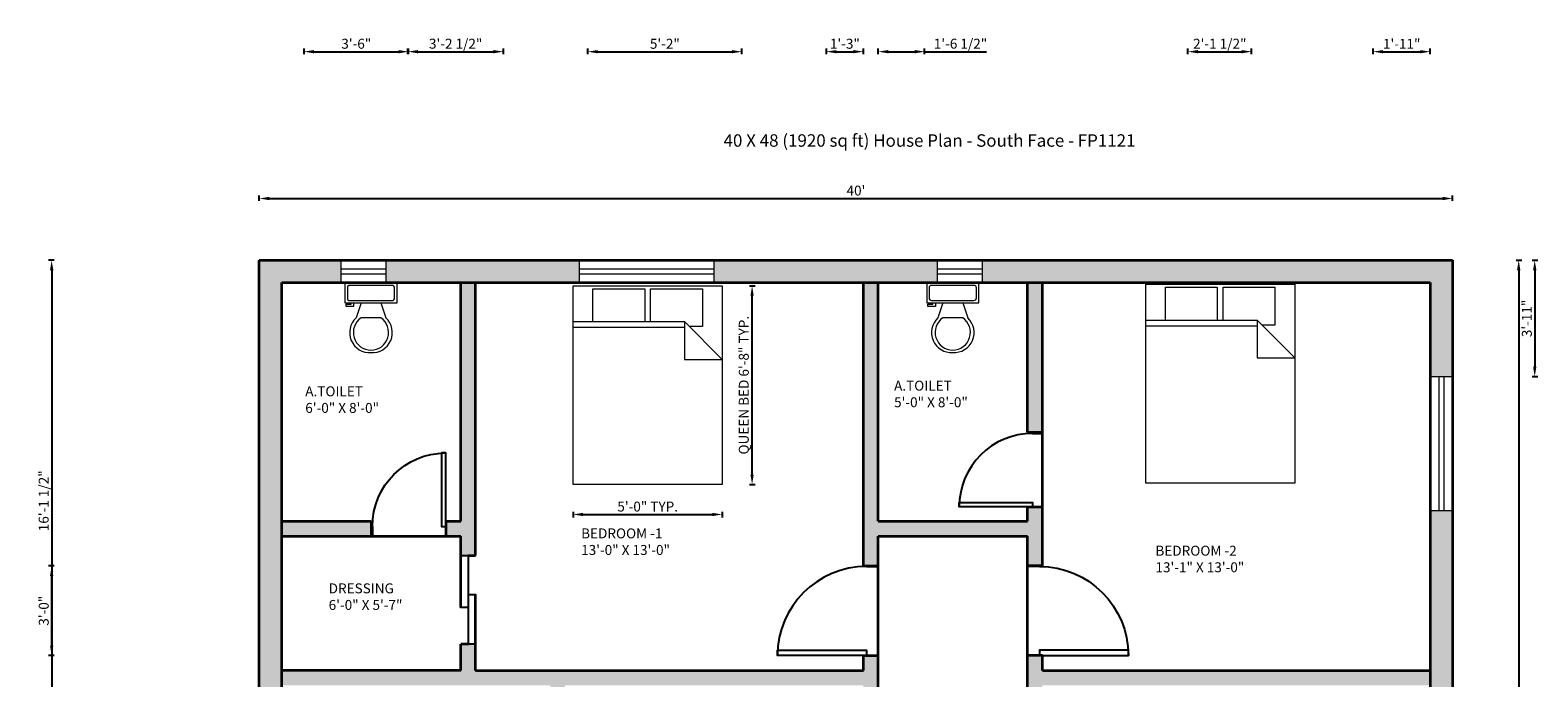
# Model space of a CAD drawing. Units: inches. Extents: x -91 to 518, y -600 to 105.
# Tile 4 of 4: x -91 to 516, y -155 to 105. Entities that reach past the tile are written whole.
import ezdxf

# ---------------------------------------------------------------- set-up
doc = ezdxf.new("R2010")
doc.units = ezdxf.units.IN
for name, color, linetype, lineweight in [('A-ANNO-DIMS', 2, 'Continuous', 18), ('A-ANNO-TITL', 7, 'Continuous', 25), ('A-AREA-IDEN', 7, 'Continuous', 18), ('A-DOOR', 4, 'Continuous', 25), ('A-FLOR-FIXT', 9, 'Continuous', 18), ('A-FURN', 8, 'Continuous', 18), ('A-GLAZ', 6, 'Continuous', 18), ('A-WALL', 7, 'Continuous', 35), ('A-WALL-PATT', 251, 'Continuous', 13)]:
    doc.layers.add(name, color=color, linetype=linetype, lineweight=lineweight)
doc.styles.get("Standard").update_dxf_attribs({"font": 'arial.ttf'})
doc.dimstyles.new('ISO-25', dxfattribs={"dimtxt": 4, "dimasz": 4, "dimexe": 1.25, "dimexo": 0.625, "dimtad": 1, "dimlunit": 3, "dimtxsty": 'Standard', "dimcen": 2.5, "dimadec": 0, "dimazin": 0, "dimtfac": 1, "dimtmove": 0, "dimatfit": 3, "dimfxl": 1, "dimfxlon": 1, "dimarcsym": 0})

# ---------------------------------------------------------------- blocks, each defined once
blk = doc.blocks.new('*U2')
for p, q in [((0, 0), (0, -100)), ((750, 0), (750, -100))]:
    blk.add_line(p, q)
blk.add_lwpolyline([(0, 0), (0, 750), (43.75, 750), (43.75, 0)], close=True)
blk.add_arc((0, 0), 750, 0, 90)
blk = doc.blocks.new('*U4')
for p, q in [((9.5, -6), (9.5, -2)), ((-10, -8.5), (-8, -8.5)), ((-10, -9.5), (-10, -8.5)), ((-7, -9.5), (-10, -9.5)), ((-8, -8.5), (-8, -8)), ((-7, -8), (-7, -9.5)), ((-4, -8), (-6, -14)), ((4, -8), (6, -14)), ((4, -14), (-4, -14))]:
    blk.add_line(p, q)
blk.add_lwpolyline([(10.5, -8), (10.5, 0), (-10.5, 0), (-10.5, -8)], close=True)
for points in [[(-9.5, -2), (-9.5, -6)], [(8.5, -1), (-8.5, -1)], [(-8.5, -7), (8.5, -7)]]:
    blk.add_lwpolyline(points)
for centre, radius, start, end in [((-8.625, -1.875), 0.8839, 81.8699, 188.1301), ((-8.625, -6.125), 0.8839, 171.869898, 278.1301), ((8.625, -1.875), 0.8839, 351.8699, 98.1301), ((8.625, -6.125), 0.8839, 261.8699, 8.1301), ((-0.4772, -19.9188), 8.0953, 133.01722, 273.38), ((0.0374, -19.8731), 7.127, 124.50543, 269.7), ((-0.0373, -19.8731), 7.127, 270.3, 55.4946), ((0.4773, -19.9188), 8.0953, 266.62, 46.9828)]:
    blk.add_arc(centre, radius, start, end)
blk = doc.blocks.new('Bed - Queen')
for p, q in [((0, -80.00003), (0, 0)), ((0, 0), (59.99999, 0)), ((59.99999, 0), (59.99999, -80.00003)), ((7.99999, -1.2), (28.79998, -1.2)), ((7.99999, -14.4), (7.99999, -1.2)), ((28.79998, -1.2), (28.79998, -14.4)), ((31.19999, -1.2), (51.99999, -1.2)), ((31.19999, -14.4), (31.19999, -1.2)), ((51.99999, -1.2), (51.99999, -16.4)), ((0, -14.4), (44.8, -14.4)), ((44.8, -16.8), (0, -16.8)), ((59.99999, -29.6), (44.8, -14.4)), ((44.8, -14.4), (44.8, -29.6)), ((51.99999, -16.4), (46.79936, -16.4)), ((44.8, -29.6), (59.99999, -29.6)), ((59.99999, -80.00003), (0, -80.00003))]:
    blk.add_line(p, q)
blk = doc.blocks.new('*D9')
at = {"layer": 'A-ANNO-DIMS', "color": 0, "lineweight": -2, "transparency": 16777216}
for p, q in [((1.54, 36.53), (1.54, 38.78)), ((5.54, 37.53), (477.54, 37.53)), ((481.54, 36.53), (481.54, 38.78))]:
    blk.add_line(p, q, dxfattribs=at)
at = {"layer": 'A-ANNO-DIMS', "color": 0, "transparency": 16777216}
for points in [[(5.54, 38.19), (5.54, 36.86), (1.54, 37.53)], [(477.54, 38.19), (477.54, 36.86), (481.54, 37.53)]]:
    blk.add_solid(points, dxfattribs=at)
at = {"layer": 'Defpoints', "color": 0, "transparency": 16777216}
for p in [(481.54, 37.53), (1.54, 12.69), (481.54, 12.69)]:
    blk.add_point(p, dxfattribs=at)
at = {"layer": 'A-ANNO-DIMS', "color": 0, "transparency": 16777216, "insert": (241.54, 40.19), "char_height": 4, "attachment_point": 5}
blk.add_mtext("40'", dxfattribs=at)
blk = doc.blocks.new('*D10')
at = {"layer": 'A-ANNO-DIMS', "color": 0, "lineweight": -2, "transparency": 16777216}
for p, q in [((507.14, 12.69), (509.39, 12.69)), ((508.14, 8.69), (508.14, -559.31)), ((507.14, -563.31), (509.39, -563.31))]:
    blk.add_line(p, q, dxfattribs=at)
at = {"layer": 'A-ANNO-DIMS', "color": 0, "transparency": 16777216}
for points in [[(507.48, 8.69), (508.81, 8.69), (508.14, 12.69)], [(507.48, -559.31), (508.81, -559.31), (508.14, -563.31)]]:
    blk.add_solid(points, dxfattribs=at)
at = {"layer": 'Defpoints', "color": 0, "transparency": 16777216}
for p in [(481.54, 12.69), (481.54, -563.31), (508.14, -563.31)]:
    blk.add_point(p, dxfattribs=at)
at = {"layer": 'A-ANNO-DIMS', "color": 0, "transparency": 16777216, "insert": (505.48, -275.31), "char_height": 4, "attachment_point": 5, "rotation": 90}
blk.add_mtext("48'", dxfattribs=at)
blk = doc.blocks.new('WIN-54IN')
for p, q in [((0, 5.5), (54, 5.5)), ((0, 3.5), (54, 3.5))]:
    blk.add_line(p, q)
blk.add_lwpolyline([(0, 9), (54, 9), (54, 0), (0, 0)], close=True)
blk = doc.blocks.new('WIN-18IN')
for p, q in [((0, 5.5), (18, 5.5)), ((0, 3.5), (18, 3.5))]:
    blk.add_line(p, q)
blk.add_lwpolyline([(0, 9), (18, 9), (18, 0), (0, 0)], close=True)
blk = doc.blocks.new('*D22')
at = {"layer": 'A-ANNO-DIMS', "color": 0, "lineweight": -2, "transparency": 16777216}
for p, q in [((198.76, 2.42), (201.01, 2.42)), ((199.76, -73.58), (199.76, -1.58)), ((198.76, -77.58), (201.01, -77.58))]:
    blk.add_line(p, q, dxfattribs=at)
at = {"layer": 'A-ANNO-DIMS', "color": 0, "transparency": 16777216}
for points in [[(199.09, -1.58), (200.42, -1.58), (199.76, 2.42)], [(199.09, -73.58), (200.42, -73.58), (199.76, -77.58)]]:
    blk.add_solid(points, dxfattribs=at)
at = {"layer": 'Defpoints', "color": 0, "transparency": 16777216}
for p in [(187.76, 2.42), (199.76, 2.42), (187.76, -77.58)]:
    blk.add_point(p, dxfattribs=at)
at = {"layer": 'A-ANNO-DIMS', "color": 0, "transparency": 16777216, "insert": (196.94, -37.58), "char_height": 4, "attachment_point": 5, "rotation": 90}
blk.add_mtext('QUEEN BED 6\'-8" TYP.', dxfattribs=at)
blk = doc.blocks.new('*D23')
at = {"layer": 'A-ANNO-DIMS', "color": 0, "lineweight": -2, "transparency": 16777216}
for p, q in [((127.76, -88.58), (127.76, -90.83)), ((131.76, -89.58), (183.76, -89.58)), ((187.76, -88.58), (187.76, -90.83))]:
    blk.add_line(p, q, dxfattribs=at)
at = {"layer": 'A-ANNO-DIMS', "color": 0, "transparency": 16777216}
for points in [[(131.76, -88.92), (131.76, -90.25), (127.76, -89.58)], [(183.76, -88.92), (183.76, -90.25), (187.76, -89.58)]]:
    blk.add_solid(points, dxfattribs=at)
at = {"layer": 'Defpoints', "color": 0, "transparency": 16777216}
for p in [(127.76, -77.58), (187.76, -77.58), (187.76, -89.58)]:
    blk.add_point(p, dxfattribs=at)
at = {"layer": 'A-ANNO-DIMS', "color": 0, "transparency": 16777216, "insert": (157.76, -86.92), "char_height": 4, "attachment_point": 5}
blk.add_mtext('5\'-0" TYP.', dxfattribs=at)
blk = doc.blocks.new('*D32')
at = {"layer": 'A-ANNO-DIMS', "color": 0, "lineweight": -2, "transparency": 16777216}
for p, q in [((19.54, 95.59), (19.54, 97.84)), ((61.54, 95.59), (61.54, 97.84)), ((23.54, 96.59), (57.54, 96.59))]:
    blk.add_line(p, q, dxfattribs=at)
at = {"layer": 'A-ANNO-DIMS', "color": 0, "transparency": 16777216}
for points in [[(23.54, 97.25), (23.54, 95.92), (19.54, 96.59)], [(57.54, 97.25), (57.54, 95.92), (61.54, 96.59)]]:
    blk.add_solid(points, dxfattribs=at)
at = {"layer": 'Defpoints', "color": 0, "transparency": 16777216}
for p in [(61.54, 96.59), (19.54, -384.72), (61.54, -384.72)]:
    blk.add_point(p, dxfattribs=at)
at = {"layer": 'A-ANNO-DIMS', "color": 0, "transparency": 16777216, "insert": (40.54, 99.26), "char_height": 4, "attachment_point": 5}
blk.add_mtext('3\'-6"', dxfattribs=at)
blk = doc.blocks.new('*D33')
at = {"layer": 'A-ANNO-DIMS', "color": 0, "lineweight": -2, "transparency": 16777216}
for p, q in [((-80.99, -110.31), (-83.24, -110.31)), ((-81.99, -142.31), (-81.99, -114.31)), ((-80.99, -146.31), (-83.24, -146.31))]:
    blk.add_line(p, q, dxfattribs=at)
at = {"layer": 'A-ANNO-DIMS', "color": 0, "transparency": 16777216}
for points in [[(-82.66, -114.31), (-81.32, -114.31), (-81.99, -110.31)], [(-82.66, -142.31), (-81.32, -142.31), (-81.99, -146.31)]]:
    blk.add_solid(points, dxfattribs=at)
at = {"layer": 'Defpoints', "color": 0, "transparency": 16777216}
for p in [(-81.99, -110.31), (310.54, -110.31), (310.54, -146.31)]:
    blk.add_point(p, dxfattribs=at)
at = {"layer": 'A-ANNO-DIMS', "color": 0, "transparency": 16777216, "insert": (-84.66, -128.31), "char_height": 4, "attachment_point": 5, "rotation": 90}
blk.add_mtext('3\'-0"', dxfattribs=at)
blk = doc.blocks.new('*D34')
at = {"layer": 'A-ANNO-DIMS', "color": 0, "lineweight": -2, "transparency": 16777216}
for p, q in [((46.54, -595.36), (46.54, -597.61)), ((50.54, -596.36), (72.54, -596.36)), ((76.54, -595.36), (76.54, -597.61))]:
    blk.add_line(p, q, dxfattribs=at)
at = {"layer": 'A-ANNO-DIMS', "color": 0, "transparency": 16777216}
for points in [[(50.54, -595.69), (50.54, -597.02), (46.54, -596.36)], [(72.54, -595.69), (72.54, -597.02), (76.54, -596.36)]]:
    blk.add_solid(points, dxfattribs=at)
at = {"layer": 'Defpoints', "color": 0, "transparency": 16777216}
for p in [(46.54, -98.31), (76.54, -98.31), (76.54, -596.36)]:
    blk.add_point(p, dxfattribs=at)
at = {"layer": 'A-ANNO-DIMS', "color": 0, "transparency": 16777216, "insert": (61.54, -593.69), "char_height": 4, "attachment_point": 5}
blk.add_mtext('2\'-6"', dxfattribs=at)
blk = doc.blocks.new('*D38')
at = {"layer": 'A-ANNO-DIMS', "color": 0, "lineweight": -2, "transparency": 16777216}
for p, q in [((449.61, 95.59), (449.61, 97.84)), ((472.54, 95.59), (472.54, 97.84)), ((453.61, 96.59), (468.54, 96.59))]:
    blk.add_line(p, q, dxfattribs=at)
at = {"layer": 'A-ANNO-DIMS', "color": 0, "transparency": 16777216}
for points in [[(453.61, 97.25), (453.61, 95.92), (449.61, 96.59)], [(468.54, 97.25), (468.54, 95.92), (472.54, 96.59)]]:
    blk.add_solid(points, dxfattribs=at)
at = {"layer": 'Defpoints', "color": 0, "transparency": 16777216}
for p in [(472.54, 96.59), (449.61, -434.96), (472.54, -434.96)]:
    blk.add_point(p, dxfattribs=at)
at = {"layer": 'A-ANNO-DIMS', "color": 0, "transparency": 16777216, "insert": (461.08, 99.22), "char_height": 4, "attachment_point": 5}
blk.add_mtext('1\'-11"', dxfattribs=at)
blk = doc.blocks.new('*D41')
at = {"layer": 'A-ANNO-DIMS', "color": 0, "lineweight": -2, "transparency": 16777216}
for p, q in [((-80.99, 12.69), (-83.24, 12.69)), ((-81.99, 8.69), (-81.99, -176.88)), ((-80.99, -180.88), (-83.24, -180.88))]:
    blk.add_line(p, q, dxfattribs=at)
at = {"layer": 'A-ANNO-DIMS', "color": 0, "transparency": 16777216}
for points in [[(-82.66, 8.69), (-81.32, 8.69), (-81.99, 12.69)], [(-82.66, -176.88), (-81.32, -176.88), (-81.99, -180.88)]]:
    blk.add_solid(points, dxfattribs=at)
at = {"layer": 'Defpoints', "color": 0, "transparency": 16777216}
for p in [(1.54, 12.69), (-81.99, -180.88), (1.54, -180.88)]:
    blk.add_point(p, dxfattribs=at)
at = {"layer": 'A-ANNO-DIMS', "color": 0, "transparency": 16777216, "insert": (-84.68, -84.09), "char_height": 4, "attachment_point": 5, "rotation": 90}
blk.add_mtext('16\'-1 1/2"', dxfattribs=at)
blk = doc.blocks.new('*D44')
at = {"layer": 'A-ANNO-DIMS', "color": 0, "lineweight": -2, "transparency": 16777216}
for p, q in [((52.46, -595.36), (52.46, -597.61)), ((56.46, -596.36), (78.54, -596.36)), ((82.54, -595.36), (82.54, -597.61))]:
    blk.add_line(p, q, dxfattribs=at)
at = {"layer": 'A-ANNO-DIMS', "color": 0, "transparency": 16777216}
for points in [[(56.46, -595.69), (56.46, -597.02), (52.46, -596.36)], [(78.54, -595.69), (78.54, -597.02), (82.54, -596.36)]]:
    blk.add_solid(points, dxfattribs=at)
at = {"layer": 'Defpoints', "color": 0, "transparency": 16777216}
for p in [(52.46, 3.69), (82.54, 3.69), (82.54, -596.36)]:
    blk.add_point(p, dxfattribs=at)
at = {"layer": 'A-ANNO-DIMS', "color": 0, "transparency": 16777216, "insert": (67.5, -593.69), "char_height": 4, "attachment_point": 5}
blk.add_mtext('2\'-6"', dxfattribs=at)
blk = doc.blocks.new('*D45')
at = {"layer": 'A-ANNO-DIMS', "color": 0, "lineweight": -2, "transparency": 16777216}
for p, q in [((88.54, -595.36), (88.54, -597.61)), ((92.54, -596.36), (126.38, -596.36)), ((130.38, -595.36), (130.38, -597.61))]:
    blk.add_line(p, q, dxfattribs=at)
at = {"layer": 'A-ANNO-DIMS', "color": 0, "transparency": 16777216}
for points in [[(92.54, -595.69), (92.54, -597.02), (88.54, -596.36)], [(126.38, -595.69), (126.38, -597.02), (130.38, -596.36)]]:
    blk.add_solid(points, dxfattribs=at)
at = {"layer": 'Defpoints', "color": 0, "transparency": 16777216}
for p in [(88.54, 3.69), (130.38, 3.69), (130.38, -596.36)]:
    blk.add_point(p, dxfattribs=at)
at = {"layer": 'A-ANNO-DIMS', "color": 0, "transparency": 16777216, "insert": (109.46, -593.69), "char_height": 4, "attachment_point": 5}
blk.add_mtext('3\'-6"', dxfattribs=at)
blk = doc.blocks.new('*D46')
at = {"layer": 'A-ANNO-DIMS', "color": 0, "lineweight": -2, "transparency": 16777216}
for p, q in [((250.54, -595.36), (250.54, -597.61)), ((254.54, -596.36), (270.34, -596.36)), ((274.34, -595.36), (274.34, -597.61))]:
    blk.add_line(p, q, dxfattribs=at)
at = {"layer": 'A-ANNO-DIMS', "color": 0, "transparency": 16777216}
for points in [[(254.54, -595.69), (254.54, -597.02), (250.54, -596.36)], [(270.34, -595.69), (270.34, -597.02), (274.34, -596.36)]]:
    blk.add_solid(points, dxfattribs=at)
at = {"layer": 'Defpoints', "color": 0, "transparency": 16777216}
for p in [(250.54, 3.69), (274.34, 3.69), (274.34, -596.36)]:
    blk.add_point(p, dxfattribs=at)
at = {"layer": 'A-ANNO-DIMS', "color": 0, "transparency": 16777216, "insert": (262.44, -593.69), "char_height": 4, "attachment_point": 5}
blk.add_mtext('2\'-0"', dxfattribs=at)
blk = doc.blocks.new('*D47')
at = {"layer": 'A-ANNO-DIMS', "color": 0, "lineweight": -2, "transparency": 16777216}
for p, q in [((513.59, 12.69), (515.84, 12.69)), ((514.59, 8.69), (514.59, -30.13)), ((513.59, -34.13), (515.84, -34.13))]:
    blk.add_line(p, q, dxfattribs=at)
at = {"layer": 'A-ANNO-DIMS', "color": 0, "transparency": 16777216}
for points in [[(513.93, 8.69), (515.26, 8.69), (514.59, 12.69)], [(513.93, -30.13), (515.26, -30.13), (514.59, -34.13)]]:
    blk.add_solid(points, dxfattribs=at)
at = {"layer": 'Defpoints', "color": 0, "transparency": 16777216}
for p in [(481.54, 12.69), (481.54, -34.13), (514.59, -34.13)]:
    blk.add_point(p, dxfattribs=at)
at = {"layer": 'A-ANNO-DIMS', "color": 0, "transparency": 16777216, "insert": (511.93, -10.72), "char_height": 4, "attachment_point": 5, "rotation": 90}
blk.add_mtext('3\'-11"', dxfattribs=at)
blk = doc.blocks.new('*D51')
at = {"layer": 'A-ANNO-DIMS', "color": 0, "lineweight": -2, "transparency": 16777216}
for p, q in [((250.54, 95.59), (250.54, 97.84)), ((269.18, 95.59), (269.18, 97.84)), ((254.54, 96.59), (265.18, 96.59)), ((269.18, 96.59), (294.01, 96.59))]:
    blk.add_line(p, q, dxfattribs=at)
at = {"layer": 'A-ANNO-DIMS', "color": 0, "transparency": 16777216}
for points in [[(254.54, 97.25), (254.54, 95.92), (250.54, 96.59)], [(265.18, 97.25), (265.18, 95.92), (269.18, 96.59)]]:
    blk.add_solid(points, dxfattribs=at)
at = {"layer": 'Defpoints', "color": 0, "transparency": 16777216}
for p in [(269.18, 96.59), (250.54, -554.31), (269.18, -554.26)]:
    blk.add_point(p, dxfattribs=at)
at = {"layer": 'A-ANNO-DIMS', "color": 0, "transparency": 16777216, "insert": (283.6, 99.28), "char_height": 4, "attachment_point": 5}
blk.add_mtext('1\'-6 1/2"', dxfattribs=at)
blk = doc.blocks.new('*D52')
at = {"layer": 'A-ANNO-DIMS', "color": 0, "lineweight": -2, "transparency": 16777216}
for p, q in [((61.33, 95.59), (61.33, 97.84)), ((99.7, 95.59), (99.7, 97.84)), ((65.33, 96.59), (95.7, 96.59))]:
    blk.add_line(p, q, dxfattribs=at)
at = {"layer": 'A-ANNO-DIMS', "color": 0, "transparency": 16777216}
for points in [[(65.33, 97.25), (65.33, 95.92), (61.33, 96.59)], [(95.7, 97.25), (95.7, 95.92), (99.7, 96.59)]]:
    blk.add_solid(points, dxfattribs=at)
at = {"layer": 'Defpoints', "color": 0, "transparency": 16777216}
for p in [(99.7, 96.59), (61.33, -393.72), (99.7, -393.72)]:
    blk.add_point(p, dxfattribs=at)
at = {"layer": 'A-ANNO-DIMS', "color": 0, "transparency": 16777216, "insert": (80.52, 99.28), "char_height": 4, "attachment_point": 5}
blk.add_mtext('3\'-2 1/2"', dxfattribs=at)
blk = doc.blocks.new('*D53')
at = {"layer": 'A-ANNO-DIMS', "color": 0, "lineweight": -2, "transparency": 16777216}
for p, q in [((133.7, 95.59), (133.7, 97.84)), ((195.65, 95.59), (195.65, 97.84)), ((137.7, 96.59), (191.65, 96.59))]:
    blk.add_line(p, q, dxfattribs=at)
at = {"layer": 'A-ANNO-DIMS', "color": 0, "transparency": 16777216}
for points in [[(137.7, 97.25), (137.7, 95.92), (133.7, 96.59)], [(191.65, 97.25), (191.65, 95.92), (195.65, 96.59)]]:
    blk.add_solid(points, dxfattribs=at)
at = {"layer": 'Defpoints', "color": 0, "transparency": 16777216}
for p in [(195.65, 96.59), (133.7, -393.72), (195.65, -393.72)]:
    blk.add_point(p, dxfattribs=at)
at = {"layer": 'A-ANNO-DIMS', "color": 0, "transparency": 16777216, "insert": (164.67, 99.25), "char_height": 4, "attachment_point": 5}
blk.add_mtext('5\'-2"', dxfattribs=at)
blk = doc.blocks.new('*D56')
at = {"layer": 'A-ANNO-DIMS', "color": 0, "lineweight": -2, "transparency": 16777216}
for p, q in [((229.65, 95.59), (229.65, 97.84)), ((244.54, 95.59), (244.54, 97.84)), ((233.65, 96.59), (240.54, 96.59))]:
    blk.add_line(p, q, dxfattribs=at)
at = {"layer": 'A-ANNO-DIMS', "color": 0, "transparency": 16777216}
for points in [[(233.65, 97.25), (233.65, 95.92), (229.65, 96.59)], [(240.54, 97.25), (240.54, 95.92), (244.54, 96.59)]]:
    blk.add_solid(points, dxfattribs=at)
at = {"layer": 'Defpoints', "color": 0, "transparency": 16777216}
for p in [(244.54, 96.59), (229.65, -384.72), (244.54, -384.72)]:
    blk.add_point(p, dxfattribs=at)
at = {"layer": 'A-ANNO-DIMS', "color": 0, "transparency": 16777216, "insert": (237.09, 99.26), "char_height": 4, "attachment_point": 5}
blk.add_mtext('1\'-3"', dxfattribs=at)
blk = doc.blocks.new('*D58')
at = {"layer": 'A-ANNO-DIMS', "color": 0, "lineweight": -2, "transparency": 16777216}
for p, q in [((375.09, 95.59), (375.09, 97.84)), ((400.72, 95.59), (400.72, 97.84)), ((379.09, 96.59), (396.72, 96.59))]:
    blk.add_line(p, q, dxfattribs=at)
at = {"layer": 'A-ANNO-DIMS', "color": 0, "transparency": 16777216}
for points in [[(379.09, 97.25), (379.09, 95.92), (375.09, 96.59)], [(396.72, 97.25), (396.72, 95.92), (400.72, 96.59)]]:
    blk.add_solid(points, dxfattribs=at)
at = {"layer": 'Defpoints', "color": 0, "transparency": 16777216}
for p in [(400.72, 96.59), (375.09, -530.31), (400.72, -533.48)]:
    blk.add_point(p, dxfattribs=at)
at = {"layer": 'A-ANNO-DIMS', "color": 0, "transparency": 16777216, "insert": (387.9, 99.28), "char_height": 4, "attachment_point": 5}
blk.add_mtext('2\'-1 1/2"', dxfattribs=at)

msp = doc.modelspace()

# ---------------------------------------------------------------- hatches: boundary and pattern name
at = {"layer": 'A-WALL-PATT'}
h = msp.add_hatch(color=256, dxfattribs=at)
h.dxf.hatch_style = 1
h.paths.add_polyline_path([(10.544, 3.693), (34.462, 3.693), (34.462, 12.693), (1.544, 12.693), (1.544, -180.878), (10.544, -180.878)])
h.paths.add_polyline_path([(46.544, -92.307), (10.544, -92.307), (10.544, -98.307), (46.544, -98.307)])
h.paths.add_polyline_path([(130.381, 12.693), (52.462, 12.693), (52.462, 3.693), (82.544, 3.693), (88.544, 3.693), (130.381, 3.693)])
h.paths.add_polyline_path([(88.544, 3.693), (82.544, 3.693), (82.544, -92.307), (76.544, -92.307), (76.544, -94.37), (76.544, -98.307), (82.544, -98.307), (82.544, -106.057), (85.522, -106.057), (88.544, -106.057)])
h.paths.add_polyline_path([(250.544, -146.307), (245.772, -146.307), (244.544, -146.307), (244.544, -152.307), (88.544, -152.307), (88.544, -141.744), (85.718, -141.744), (82.544, -141.744), (82.544, -152.307), (10.544, -152.307), (10.544, -158.307), (88.544, -158.307), (118.544, -158.307), (118.544, -164.307), (120.607, -164.307), (124.544, -164.307), (124.544, -158.307), (244.544, -158.307), (244.544, -164.307), (250.544, -164.307)])
h.paths.add_polyline_path([(274.341, 12.693), (184.381, 12.693), (184.381, 3.693), (244.544, 3.693), (250.544, 3.693), (274.341, 3.693)])
h.paths.add_polyline_path([(250.544, 3.693), (244.544, 3.693), (244.544, -110.307), (250.544, -110.307), (250.544, -98.307), (310.544, -98.307), (310.544, -110.307), (316.544, -110.307), (316.544, -86.517), (312.607, -86.517), (310.544, -86.517), (310.544, -92.307), (250.544, -92.307)])
h.paths.add_polyline_path([(481.544, 12.693), (292.341, 12.693), (292.341, 3.693), (310.544, 3.693), (316.544, 3.693), (472.544, 3.693), (472.544, -34.129), (481.544, -34.129)])
h.paths.add_polyline_path([(316.544, 3.693), (310.544, 3.693), (310.544, -56.517), (316.544, -56.517)], flags=17)
h.paths.add_polyline_path([(481.544, -88.129), (472.544, -88.129), (472.544, -189.451), (481.544, -189.451)])
h.paths.add_polyline_path([(472.544, -152.307), (316.544, -152.307), (316.544, -146.307), (315.319, -146.307), (310.544, -146.307), (310.544, -260.307), (316.544, -260.307), (316.544, -158.307), (472.544, -158.307)])
h.paths.add_polyline_path([(481.544, -243.451), (472.544, -243.451), (472.544, -308.307), (472.544, -332.593), (481.544, -332.593)])
h.paths.add_polyline_path([(472.544, -302.307), (316.544, -302.307), (316.544, -296.307), (315.322, -296.307), (310.544, -296.307), (310.544, -308.307), (472.544, -308.307)])
h.paths.add_polyline_path([(481.544, -366.593), (472.544, -366.593), (472.544, -385.307), (472.544, -456.136), (481.544, -456.136)])
h.paths.add_polyline_path([(472.544, -385.307), (310.544, -385.307), (310.544, -391.307), (472.544, -391.307)])
h.paths.add_polyline_path([(481.544, -510.136), (472.544, -510.136), (472.544, -554.307), (323.185, -554.307), (323.185, -563.307), (481.544, -563.307)])
h.paths.add_polyline_path([(250.544, -384.724), (229.645, -384.724), (229.645, -393.724), (241.544, -393.724), (241.544, -563.307), (269.185, -563.307), (269.185, -554.307), (250.544, -554.307)])
h.paths.add_polyline_path([(195.645, -384.724), (133.7, -384.724), (133.7, -393.724), (195.645, -393.724)])
h.paths.add_polyline_path([(99.7, -384.724), (61.544, -384.724), (61.544, -391.562), (61.335, -393.724), (77.042, -393.724), (99.7, -393.724)])
h.paths.add_polyline_path([(10.544, -264.014), (1.544, -264.014), (1.544, -330.048), (10.544, -330.048)])
h.paths.add_polyline_path([(10.544, -198.878), (1.544, -198.878), (1.544, -230.014), (10.544, -230.014)])
h.paths.add_polyline_path([(208.544, -218.307), (124.544, -218.307), (124.544, -194.307), (118.544, -194.307), (118.544, -218.307), (10.544, -218.307), (10.544, -224.307), (118.544, -224.307), (124.544, -224.307), (208.544, -224.307)])
h.paths.add_polyline_path([(250.544, -194.307), (244.544, -194.307), (244.544, -218.307), (238.544, -218.307), (238.544, -224.307), (244.544, -224.307), (244.544, -384.724), (250.544, -384.724)])

# ---------------------------------------------------------------- linework, layer by layer
at = {"layer": 'A-DOOR'}
for points in [[(82.544, -106.057), (85.522, -106.057), (85.522, -127.048), (82.544, -127.048)], [(85.718, -121.823), (88.544, -121.823), (88.544, -141.744), (85.718, -141.744)]]:
    msp.add_lwpolyline(points, close=True, dxfattribs=at)
at = {"layer": 'A-WALL'}
for p, q in [((1.544, 12.693), (481.544, 12.693)), ((1.544, -563.307), (1.544, 12.693)), ((481.544, 12.693), (481.544, -563.307)), ((10.544, 3.693), (82.544, 3.693)), ((10.544, -384.724), (10.544, 3.693)), ((82.544, 3.693), (88.544, 3.693)), ((82.544, -92.307), (82.544, 3.693)), ((88.544, 3.693), (244.544, 3.693)), ((88.544, -106.057), (88.544, 3.693)), ((244.544, 3.693), (250.544, 3.693)), ((244.544, -110.307), (244.544, 3.693)), ((250.544, 3.693), (310.544, 3.693)), ((250.544, -92.307), (250.544, 3.693)), ((310.544, 3.693), (316.544, 3.693)), ((310.544, -56.517), (310.544, 3.693)), ((316.544, 3.693), (472.544, 3.693)), ((316.544, -110.307), (316.544, 3.693)), ((472.544, 3.693), (472.544, -308.307)), ((310.544, -56.517), (316.544, -56.517)), ((310.544, -86.517), (316.544, -86.517)), ((310.544, -92.307), (310.544, -86.517)), ((10.544, -92.307), (46.544, -92.307)), ((46.544, -92.307), (46.544, -98.307)), ((76.544, -92.307), (76.544, -98.307)), ((76.544, -92.307), (82.544, -92.307)), ((250.544, -92.307), (310.544, -92.307)), ((10.544, -98.307), (82.544, -98.307)), ((82.544, -127.048), (82.544, -98.307)), ((250.544, -98.307), (310.544, -98.307)), ((250.544, -164.307), (250.544, -98.307)), ((310.544, -308.307), (310.544, -98.307)), ((85.522, -106.057), (88.544, -106.057)), ((244.544, -110.307), (250.544, -110.307)), ((316.544, -110.307), (310.544, -110.307)), ((88.544, -152.307), (88.544, -121.823)), ((82.544, -152.307), (82.544, -141.744)), ((85.718, -141.744), (82.544, -141.744)), ((244.544, -146.307), (250.544, -146.307)), ((244.544, -152.307), (244.544, -146.307)), ((316.544, -146.307), (310.544, -146.307)), ((316.544, -152.307), (316.544, -146.307)), ((82.544, -152.307), (10.544, -152.307)), ((88.544, -152.307), (244.544, -152.307)), ((316.544, -152.307), (472.544, -152.307))]:
    msp.add_line(p, q, dxfattribs=at)

# ---------------------------------------------------------------- block references
at = {"layer": 'A-DOOR'}
for p, xscale, yscale, zscale, rotation in [((312.607, -86.517), 0.0393700787401575, 0.0393700787401575, 0.0393700787401575, 90), ((245.772, -146.307), 0.0477231779789571, 0.0477231779789571, 0.0477231779789571, 90), ((315.319, -146.307), -0.0477503836946777, 0.0477503836946777, 0.0477503836946777, 270)]:
    msp.add_blockref('*U2', p, dxfattribs=dict(at, xscale=xscale, yscale=yscale, zscale=zscale, rotation=rotation))
at = {"layer": 'A-DOOR', "xscale": -0.0393700787401575, "yscale": 0.0393700787401575, "zscale": 0.0393700787401575}
msp.add_blockref('*U2', (76.544, -94.37), dxfattribs=at)
at = {"layer": 'A-FLOR-FIXT'}
for p in [(46.458, 3.513), (280.498, 3.538)]:
    msp.add_blockref('*U4', p, dxfattribs=at)
at = {"layer": 'A-FURN'}
for p in [(127.756, 2.416), (358.095, 3.031)]:
    msp.add_blockref('Bed - Queen', p, dxfattribs=at)
at = {"layer": 'A-GLAZ'}
for name, p in [('WIN-18IN', (34.462, 3.693)), ('WIN-54IN', (130.381, 3.688)), ('WIN-18IN', (274.341, 3.693))]:
    msp.add_blockref(name, p, dxfattribs=at)
at = {"layer": 'A-GLAZ', "rotation": 269.9999999999999}
msp.add_blockref('WIN-54IN', (472.544, -34.13), dxfattribs=at)
msp.add_blockref('WIN-54IN', (472.544, -34.13), dxfattribs=at)

# ---------------------------------------------------------------- texts
at = {"layer": 'A-ANNO-TITL', "insert": (188.293, 63.356), "char_height": 5, "attachment_point": 1}
msp.add_mtext_dynamic_manual_height_columns('40 X 48 (1920 sq ft) House Plan - South Face - FP1121', width=415.95292, gutter_width=12.5, heights=[0], dxfattribs=at)
at = {"layer": 'A-AREA-IDEN', "char_height": 4, "attachment_point": 1}
for s, width, insert in [('A.TOILET\\P5\'-0" X 8\'-0"', 44.87593, (256.878, -35.764)), ('A.TOILET\\P6\'-0" X 8\'-0"', 47.53268, (20.017, -38.047)), ('BEDROOM -1\\P13\'-0" X 13\'-0"', 75.28852, (130.998, -95.193)), ('BEDROOM -2\\P13\'-1" X 13\'-0"', 88.25728, (362.013, -102.157)), ('DRESSING\\P6\'-0" X 5\'-7"', 55.27588, (29.433, -117.312))]:
    msp.add_mtext_dynamic_manual_height_columns(s, width=width, gutter_width=12.5, heights=[0], dxfattribs=dict(at, insert=insert))

# ---------------------------------------------------------------- dimensions: what is measured, and where the dimension line sits
at = {"layer": 'A-ANNO-DIMS'}
for base, p1, p2, override, picture, middle in [((99.7, 96.588), (61.335, -393.724), (99.7, -393.724), {"dimdec": 1, "dimlfac": 1, "dimrnd": 0, "dimzin": 1, "dimdsep": 46, "dimlunit": 4, "dimfrac": 2}, '*D52', (80.518, 99.282)), ((269.185, 96.588), (250.544, -554.307), (269.185, -554.258), {"dimdec": 1, "dimlfac": 1, "dimrnd": 0, "dimzin": 1, "dimdsep": 46, "dimlunit": 4, "dimfrac": 2}, '*D51', (283.598, 99.281)), ((400.722, 96.588), (375.087, -530.307), (400.722, -533.48), {"dimdec": 1, "dimlfac": 1, "dimrnd": 0, "dimzin": 1, "dimdsep": 46, "dimlunit": 4, "dimfrac": 2}, '*D58', (387.904, 99.281)), ((61.544, 96.588), (19.544, -384.724), (61.544, -384.724), {"dimdec": 1, "dimlfac": 1, "dimrnd": 0, "dimzin": 1, "dimdsep": 46, "dimlunit": 4, "dimfrac": 2}, '*D32', (40.544, 99.256)), ((195.645, 96.588), (133.7, -393.724), (195.645, -393.724), {"dimdec": 1, "dimlfac": 1, "dimrnd": 0, "dimzin": 1, "dimdsep": 46, "dimlunit": 4, "dimfrac": 2}, '*D53', (164.673, 99.255)), ((244.544, 96.588), (229.645, -384.724), (244.544, -384.724), {"dimdec": 1, "dimlfac": 1, "dimrnd": 0, "dimzin": 1, "dimdsep": 46, "dimlunit": 4, "dimfrac": 2}, '*D56', (237.095, 99.256)), ((472.544, 96.588), (449.608, -434.957), (472.544, -434.957), {"dimdec": 1, "dimlfac": 1, "dimrnd": 0, "dimzin": 1, "dimdsep": 46, "dimlunit": 4, "dimfrac": 2}, '*D38', (461.076, 99.221)), ((481.544, 37.525), (1.544, 12.693), (481.544, 12.693), {"dimclrd": 0, "dimclre": 0, "dimclrt": 0}, '*D9', (241.544, 40.193)), ((82.544, -596.357), (52.462, 3.693), (82.544, 3.693), {"dimdec": 1, "dimlfac": 1, "dimrnd": 0, "dimzin": 1, "dimdsep": 46, "dimlunit": 4, "dimfrac": 2}, '*D44', (67.503, -593.69)), ((130.381, -596.357), (88.544, 3.693), (130.381, 3.688), {"dimdec": 1, "dimlfac": 1, "dimrnd": 0, "dimzin": 1, "dimdsep": 46, "dimlunit": 4, "dimfrac": 2}, '*D45', (109.462, -593.688)), ((274.341, -596.357), (250.544, 3.693), (274.341, 3.693), {"dimdec": 1, "dimlfac": 1, "dimrnd": 0, "dimzin": 1, "dimdsep": 46, "dimlunit": 4, "dimfrac": 2}, '*D46', (262.442, -593.69)), ((76.544, -596.357), (46.544, -98.307), (76.544, -98.307), {"dimdec": 1, "dimlfac": 1, "dimrnd": 0, "dimzin": 1, "dimdsep": 46, "dimlunit": 4, "dimfrac": 2}, '*D34', (61.544, -593.69))]:
    dim = msp.add_linear_dim(base=base, p1=p1, p2=p2, dimstyle='ISO-25', override=override, dxfattribs=at)
    dim.commit()
    dim.dimension.update_dxf_attribs({"geometry": picture, "text_midpoint": middle})
for base, p1, p2, override, picture, middle in [((-81.989, -180.878), (1.544, 12.693), (1.544, -180.878), {"dimdec": 1, "dimlfac": 1, "dimrnd": 0, "dimzin": 1, "dimdsep": 46, "dimlunit": 4, "dimfrac": 2}, '*D41', (-84.682, -84.092)), ((508.145, -563.307), (481.544, 12.693), (481.544, -563.307), {"dimclrd": 0, "dimclre": 0, "dimclrt": 0}, '*D10', (505.477, -275.307)), ((514.594, -34.129), (481.544, 12.693), (481.544, -34.129), {"dimdec": 1, "dimlfac": 1, "dimrnd": 0, "dimzin": 1, "dimdsep": 46, "dimlunit": 4, "dimfrac": 2}, '*D47', (511.925, -10.718)), ((-81.989, -110.307), (310.544, -146.307), (310.544, -110.307), {"dimdec": 1, "dimlfac": 1, "dimrnd": 0, "dimzin": 1, "dimdsep": 46, "dimlunit": 4, "dimfrac": 2}, '*D33', (-84.657, -128.307))]:
    dim = msp.add_linear_dim(base=base, p1=p1, p2=p2, angle=90, dimstyle='ISO-25', override=override, dxfattribs=at)
    dim.commit()
    dim.dimension.update_dxf_attribs({"geometry": picture, "text_midpoint": middle})
dim = msp.add_linear_dim(base=(199.756, 2.416), p1=(187.756, -77.585), p2=(187.756, 2.416), angle=90, text='QUEEN BED <> TYP.', dimstyle='ISO-25', override={"dimdec": 1, "dimlfac": 1, "dimrnd": 0, "dimzin": 1, "dimdsep": 46, "dimlunit": 4, "dimfrac": 2}, dxfattribs=at)
dim.commit()
dim.dimension.update_dxf_attribs({"geometry": '*D22', "text_midpoint": (196.94, -37.584)})
dim = msp.add_linear_dim(base=(187.756, -89.585), p1=(127.756, -77.585), p2=(187.756, -77.585), text='<> TYP.', dimstyle='ISO-25', override={"dimdec": 1, "dimlfac": 1, "dimrnd": 0, "dimzin": 1, "dimdsep": 46, "dimlunit": 4, "dimfrac": 2}, dxfattribs=at)
dim.commit()
dim.dimension.update_dxf_attribs({"geometry": '*D23', "text_midpoint": (157.756, -86.917)})

doc.saveas('drawing.dxf')
